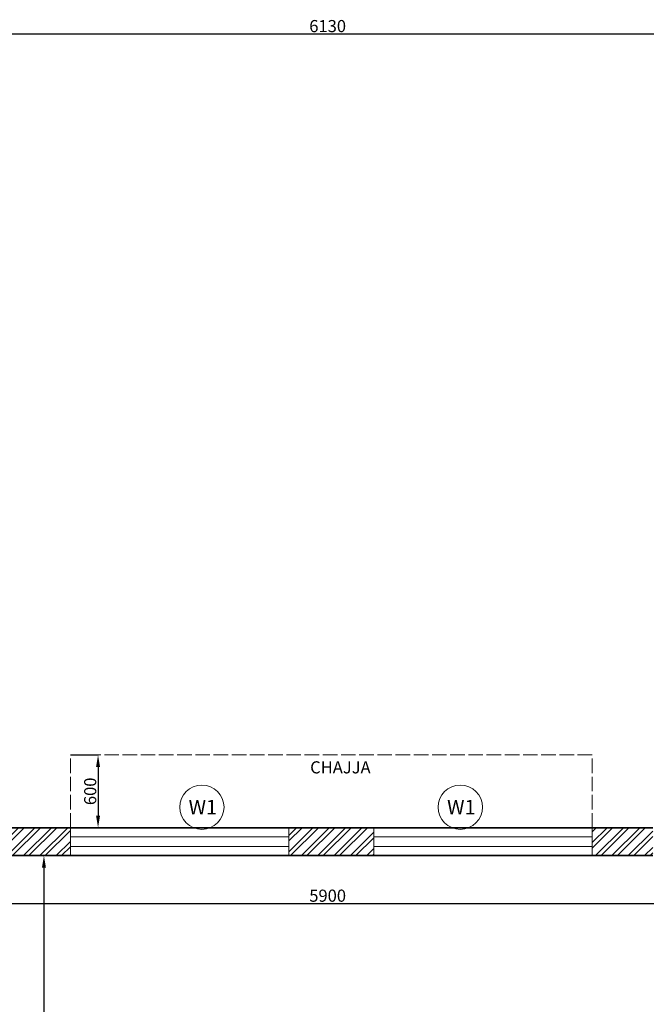
# Model space of a CAD drawing. Units: millimetres. Extents: x -3326 to 29338, y -16792 to 6002.
# Tile 12 of 21: x 11795 to 16958, y -3440 to 4678. Entities that reach past the tile are written whole.
import ezdxf

# ---------------------------------------------------------------- set-up
doc = ezdxf.new("R2010")
doc.units = ezdxf.units.MM
doc.header["$PDMODE"] = 35
doc.header["$PDSIZE"] = 5
doc.linetypes.add('ACAD_ISO02W100', pattern=[15, 12, -3])
for name, color, linetype, lineweight in [('A-ANNO-DIMS', 2, 'Continuous', 13), ('A-ANNO-SYMB', 7, 'Continuous', 18), ('A-GLAZ', 4, 'Continuous', 18), ('A-ROOF-OVHD', 8, 'ACAD_ISO02W100', 13), ('A-WALL', 7, 'Continuous', 35), ('A-WALL-PATT', 252, 'Continuous', 13), ('txt', 7, 'Continuous', 18)]:
    doc.layers.add(name, color=color, linetype=linetype, lineweight=lineweight)
doc.styles.get("Standard").update_dxf_attribs({"font": 'arial.ttf'})
doc.dimstyles.new('ISO-25', dxfattribs={"dimtxt": 100, "dimasz": 100, "dimexe": 1.25, "dimexo": 0.625, "dimtad": 1, "dimtxsty": 'Standard', "dimcen": 2.5, "dimadec": 0, "dimazin": 0, "dimtfac": 1, "dimtmove": 0, "dimatfit": 3, "dimfxl": 1, "dimarcsym": 0})

# ---------------------------------------------------------------- blocks, each defined once
blk = doc.blocks.new('*D49')
at = {"layer": 'A-ANNO-DIMS', "color": 0, "lineweight": -2, "transparency": 16777216}
for p, q in [((12018.3, -2214), (11993.3, -2214)), ((11994.5, -2314), (11994.5, -6350.4)), ((11995.1, -6450.4), (11995.8, -6450.4))]:
    blk.add_line(p, q, dxfattribs=at)
at = {"layer": 'A-ANNO-DIMS', "color": 0, "transparency": 16777216}
for points in [[(11977.9, -2314), (12011.2, -2314), (11994.5, -2214)], [(11977.9, -6350.4), (12011.2, -6350.4), (11994.5, -6450.4)]]:
    blk.add_solid(points, dxfattribs=at)
at = {"layer": 'Defpoints', "color": 0, "transparency": 16777216}
for p in [(12018.9, -2214), (11994.5, -6450.4), (11994.5, -6450.4)]:
    blk.add_point(p, dxfattribs=at)
at = {"layer": 'A-ANNO-DIMS', "color": 0, "transparency": 16777216, "insert": (11933.8, -4332.2), "char_height": 100, "attachment_point": 5, "rotation": 90}
blk.add_mtext('4236,45', dxfattribs=at)
blk = doc.blocks.new('*D50')
at = {"layer": 'A-ANNO-DIMS', "color": 0, "lineweight": -2, "transparency": 16777216}
for p, q in [((11382.3, -2608.3), (11382.3, -2607.7)), ((11482.3, -2609), (17182.3, -2609)), ((17282.3, -2608.3), (17282.3, -2607.7))]:
    blk.add_line(p, q, dxfattribs=at)
at = {"layer": 'A-ANNO-DIMS', "color": 0, "transparency": 16777216}
for points in [[(11482.3, -2592.3), (11482.3, -2625.6), (11382.3, -2609)], [(17182.3, -2592.3), (17182.3, -2625.6), (17282.3, -2609)]]:
    blk.add_solid(points, dxfattribs=at)
at = {"layer": 'Defpoints', "color": 0, "transparency": 16777216}
for p in [(11382.3, -2609), (17282.3, -2609), (17282.3, -2609)]:
    blk.add_point(p, dxfattribs=at)
at = {"layer": 'A-ANNO-DIMS', "color": 0, "transparency": 16777216, "insert": (14332.3, -2557.3), "char_height": 100, "attachment_point": 5}
blk.add_mtext('5900', dxfattribs=at)
blk = doc.blocks.new('*D53')
at = {"layer": 'A-ANNO-DIMS', "color": 0, "lineweight": -2, "transparency": 16777216}
for p, q in [((12212.9, -1384), (12441.6, -1384)), ((12440.3, -1484), (12440.3, -1884)), ((12212.9, -1984), (12441.6, -1984))]:
    blk.add_line(p, q, dxfattribs=at)
at = {"layer": 'A-ANNO-DIMS', "color": 0, "transparency": 16777216}
for points in [[(12423.7, -1484), (12457, -1484), (12440.3, -1384)], [(12423.7, -1884), (12457, -1884), (12440.3, -1984)]]:
    blk.add_solid(points, dxfattribs=at)
at = {"layer": 'Defpoints', "color": 0, "transparency": 16777216}
for p in [(12212.3, -1384), (12212.3, -1984), (12440.3, -1984)]:
    blk.add_point(p, dxfattribs=at)
at = {"layer": 'A-ANNO-DIMS', "color": 0, "transparency": 16777216, "insert": (12388.7, -1684), "char_height": 100, "attachment_point": 5, "rotation": 90}
blk.add_mtext('600', dxfattribs=at)
blk = doc.blocks.new('*D154')
at = {"layer": 'A-ANNO-DIMS', "color": 0, "lineweight": -2, "transparency": 16777216}
for p, q in [((11267.3, 4562.4), (11267.3, 4559.3)), ((11367.3, 4560.5), (17297.3, 4560.5)), ((17397.3, 4561.1), (17397.3, 4561.8))]:
    blk.add_line(p, q, dxfattribs=at)
at = {"layer": 'A-ANNO-DIMS', "color": 0, "transparency": 16777216}
for points in [[(11367.3, 4577.2), (11367.3, 4543.8), (11267.3, 4560.5)], [(17297.3, 4577.2), (17297.3, 4543.8), (17397.3, 4560.5)]]:
    blk.add_solid(points, dxfattribs=at)
at = {"layer": 'Defpoints', "color": 0, "transparency": 16777216}
for p in [(11267.3, 4563), (17397.3, 4560.5), (17397.3, 4560.5)]:
    blk.add_point(p, dxfattribs=at)
at = {"layer": 'A-ANNO-DIMS', "color": 0, "transparency": 16777216, "insert": (14332.3, 4612.2), "char_height": 100, "attachment_point": 5}
blk.add_mtext('6130', dxfattribs=at)
blk = doc.blocks.new('TAG-W1')
blk.add_circle((182.6, 182.6), 182.6)
at = {"insert": (73.3, 242.9), "char_height": 120, "attachment_point": 1}
blk.add_mtext_dynamic_manual_height_columns('W1', width=232.46, gutter_width=12.5, heights=[0], dxfattribs=at)
blk = doc.blocks.new('GLAZ-1800x80')
for p, q in [((0, 80), (1800, 80)), ((0, 0), (1800, 0))]:
    blk.add_line(p, q)

msp = doc.modelspace()

# ---------------------------------------------------------------- hatches: boundary and pattern name
at = {"layer": 'A-WALL-PATT'}
h = msp.add_hatch(dxfattribs=at)
h.set_pattern_fill('ANSI32', color=256, scale=10)
h.set_pattern_definition([(45, (-10476.65, 1e-12), (-67.35192, 67.35192), []), (45, (-10431.74, 1e-12), (-67.35192, 67.35192), [])])
h.paths.add_polyline_path([(12212.301, -1983.952), (11640.861, -1983.952), (11640.861, -2213.952), (12212.301, -2213.952)])
h.paths.add_polyline_path([(14712.301, -1983.952), (14012.301, -1983.952), (14012.301, -2213.952), (14712.301, -2213.952)])
h.paths.add_polyline_path([(17012.301, -1983.952), (16512.301, -1983.952), (16512.301, -2213.952), (17012.301, -2213.952)])
h.paths.add_polyline_path([(11382.301, -2383.952), (11040.861, -2383.952), (7302.301, -2383.952), (7302.301, -1935.766), (7217.026, -1935.766), (7202.301, -1933.952), (7202.301, -2483.952), (7302.301, -2483.952), (11152.301, -2483.952), (11152.301, -2833.952), (11283.549, -2833.952), (11283.549, -2830.395), (11363.875, -2830.395), (11382.301, -2833.952)])
h.paths.add_polyline_path([(11382.301, -3733.952), (11363.875, -3733.952), (11363.875, -3734.058), (11283.549, -3734.058), (11152.301, -3733.952), (11152.301, -6450.401), (11382.301, -6450.401)])
h.paths.add_polyline_path([(13462.301, -6450.401), (12606.738, -6450.401), (11382.301, -6450.401), (11382.301, -6680.401), (12606.738, -6680.401), (13462.301, -6680.401)])
h.paths.add_polyline_path([(11382.301, -7050.401), (11152.301, -7050.401), (11152.301, -8810.401), (11382.301, -8810.401)])
h.paths.add_polyline_path([(13462.301, -8980.401), (11751.174, -8980.401), (11751.174, -9210.401), (13462.301, -9210.401)])
h.paths.add_polyline_path([(13962.301, -6850.401), (13732.301, -6850.401), (13732.301, -7350.401), (13962.301, -7350.401)])
h.paths.add_polyline_path([(13962.301, -8309.482), (13732.301, -8309.482), (13732.301, -8809.482), (13962.301, -8809.482)])
h.paths.add_polyline_path([(15712.301, -12533.952), (12902.301, -12533.952), (12902.301, -12763.952), (15712.301, -12763.952)])
h.paths.add_polyline_path([(11508.301, -9211.585), (11382.301, -9211.585), (11152.301, -9211.585), (11152.301, -11033.952), (10952.301, -11033.952), (10952.301, -11263.952), (11152.301, -11263.952), (11152.301, -12361.585), (11508.301, -12361.585)])
h.paths.add_polyline_path([(12002.301, -12533.952), (11902.301, -12533.952), (11902.301, -12761.585), (11152.301, -12761.585), (11152.301, -12763.952), (11902.301, -12763.952), (12002.301, -12763.952)])
h.paths.add_polyline_path([(17112.301, -12533.952), (16912.301, -12533.952), (16912.301, -12763.952), (17112.301, -12763.952)])
h.paths.add_polyline_path([(11382.301, 3596.048), (11152.301, 3596.048), (11152.301, 2096.048), (11382.301, 2096.048)])
h.paths.add_polyline_path([(11382.301, 1496.048), (11152.301, 1496.048), (11152.301, -1983.952), (11382.301, -1983.952)])

# ---------------------------------------------------------------- linework, layer by layer
at = {"layer": 'A-GLAZ'}
for p, q in [((12212.301, -1983.952), (12212.301, -2213.952)), ((14012.301, -1983.952), (14012.301, -2213.952)), ((14712.301, -1983.952), (14712.301, -2213.952)), ((16512.301, -1983.952), (16512.301, -2213.952))]:
    msp.add_line(p, q, dxfattribs=at)
at = {"layer": 'A-ROOF-OVHD', "ltscale": 10}
for p, q in [((12212.301, -1983.952), (12212.301, -1383.952)), ((16512.301, -1383.952), (12212.301, -1383.952)), ((16512.301, -1983.952), (16512.301, -1383.952))]:
    msp.add_line(p, q, dxfattribs=at)
at = {"layer": 'A-WALL'}
for p, q in [((17012.301, -1983.952), (11640.861, -1983.952)), ((17012.301, -2213.952), (11640.861, -2213.952))]:
    msp.add_line(p, q, dxfattribs=at)

# ---------------------------------------------------------------- block references
at = {"layer": 'A-ANNO-SYMB'}
for p in [(13113.282, -1997.42), (15242.951, -1997.42)]:
    msp.add_blockref('TAG-W1', p, dxfattribs=at)
at = {"layer": 'A-GLAZ'}
for p in [(12212.301, -2138.952), (14712.301, -2138.952)]:
    msp.add_blockref('GLAZ-1800x80', p, dxfattribs=at)

# ---------------------------------------------------------------- texts
at = {"layer": 'txt', "insert": (14188.162, -1436.244), "char_height": 100, "attachment_point": 1}
msp.add_mtext_dynamic_manual_height_columns('CHAJJA', width=659.30637, gutter_width=12.5, heights=[0], dxfattribs=at)

# ---------------------------------------------------------------- dimensions: what is measured, and where the dimension line sits
at = {"layer": 'A-ANNO-DIMS'}
for base, p1, p2, picture, middle in [((17397.301, 4560.514), (11267.301, 4563.014), (17397.301, 4560.514), '*D154', (14332.301, 4612.231)), ((17282.301, -2608.952), (11382.301, -2608.952), (17282.301, -2608.952), '*D50', (14332.301, -2557.27))]:
    dim = msp.add_linear_dim(base=base, p1=p1, p2=p2, dimstyle='ISO-25', override={"dimclrd": 0, "dimclre": 0, "dimclrt": 0}, dxfattribs=at)
    dim.commit()
    dim.dimension.update_dxf_attribs({"geometry": picture, "text_midpoint": middle})
for base, p1, p2, picture, middle in [((12440.34, -1983.952), (12212.301, -1383.952), (12212.301, -1983.952), '*D53', (12388.658, -1683.952)), ((11994.519, -6450.401), (12018.923, -2213.952), (11994.519, -6450.401), '*D49', (11933.799, -4332.177))]:
    dim = msp.add_linear_dim(base=base, p1=p1, p2=p2, angle=90, dimstyle='ISO-25', override={"dimclrd": 0, "dimclre": 0, "dimclrt": 0}, dxfattribs=at)
    dim.commit()
    dim.dimension.update_dxf_attribs({"geometry": picture, "text_midpoint": middle})

doc.saveas('drawing.dxf')
